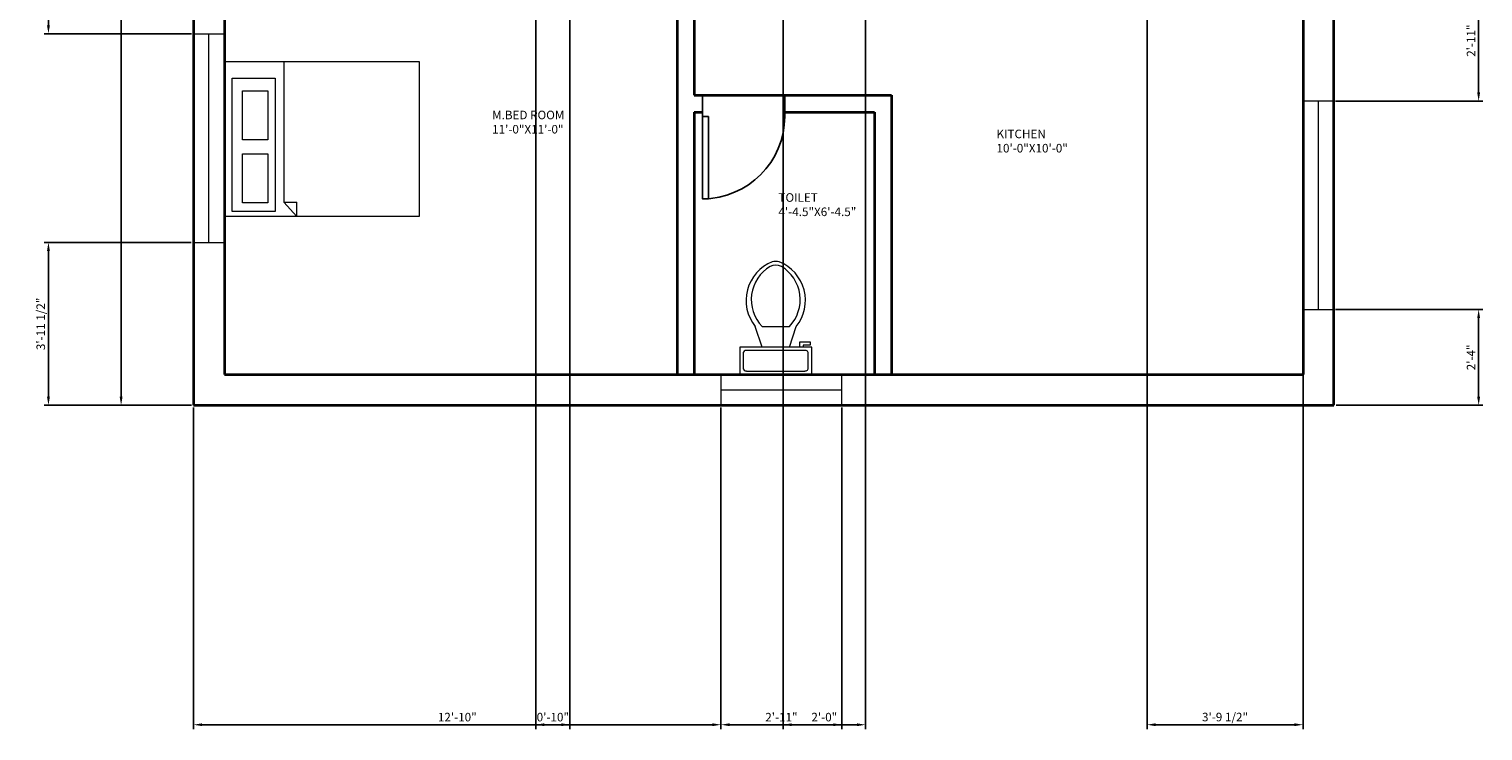
# Model space of a CAD drawing. Units: inches. Extents: x 4673 to 5097, y 7020 to 7947.
# Tile 1 of 3: x 4673 to 5097, y 7020 to 7225. Entities that reach past the tile are written whole.
import ezdxf

# ---------------------------------------------------------------- set-up
doc = ezdxf.new("R2010")
doc.units = ezdxf.units.IN
for name, color, linetype, lineweight in [('A-ANNO-DIMS', 244, 'Continuous', 18), ('A-AREA-IDEN', 7, 'Continuous', 18), ('A-DOOR', 4, 'Continuous', 25), ('A-FLOR-FIXT', 8, 'Continuous', 18), ('A-FURN', 152, 'Continuous', 18), ('A-GLAZ', 152, 'Continuous', 18), ('A-WALL', 7, 'Continuous', 35)]:
    doc.layers.add(name, color=color, linetype=linetype, lineweight=lineweight)
doc.styles.get("Standard").update_dxf_attribs({"font": 'arial.ttf'})
doc.dimstyles.new('ISO-25', dxfattribs={"dimtxt": 2.5, "dimasz": 2.5, "dimexe": 1.25, "dimexo": 0.625, "dimtad": 1, "dimlunit": 3, "dimtxsty": 'Standard', "dimcen": 2.5, "dimadec": 0, "dimazin": 0, "dimtfac": 1, "dimtmove": 0, "dimatfit": 3, "dimfxl": 1, "dimarcsym": 0})

# ---------------------------------------------------------------- blocks, each defined once
blk = doc.blocks.new('*U6')
for p, q in [((-24, 0), (-24, -6)), ((0, 0), (0, -6))]:
    blk.add_line(p, q)
blk.add_lwpolyline([(0, 0), (0, 24), (-1.75, 24), (-1.75, 0)], close=True)
blk.add_arc((0, 0), 24, 90, 180)
blk = doc.blocks.new('*U8')
for p, q in [((9.5, -6), (9.5, -2)), ((-8, -8.5), (-8, -8)), ((-7, -8), (-7, -9.5)), ((-4, -8), (-6, -14)), ((4, -8), (6, -14)), ((-10, -8.5), (-8, -8.5)), ((-10, -9.5), (-10, -8.5)), ((-7, -9.5), (-10, -9.5)), ((4, -14), (-4, -14))]:
    blk.add_line(p, q)
blk.add_lwpolyline([(10.5, -8), (10.5, 0), (-10.5, 0), (-10.5, -8)], close=True)
for points in [[(-9.5, -2), (-9.5, -6)], [(8.5, -1), (-8.5, -1)], [(-8.5, -7), (8.5, -7)]]:
    blk.add_lwpolyline(points)
for centre, radius, start, end in [((-8.62, -1.88), 0.884, 81.8699, 188.1301), ((8.62, -1.88), 0.884, 351.8699, 98.1301), ((-8.62, -6.12), 0.884, 171.8699, 278.1301), ((8.62, -6.12), 0.884, 261.8699, 8.1301), ((3.52, -21.58), 12.17, 141.4691, 247.9714), ((4.2, -21.82), 11.33, 136.3677, 238.9468), ((-3.52, -21.58), 12.17, 292.0284, 38.5307), ((-4.2, -21.82), 11.33, 301.053, 43.6321), ((0, -27.88), 4, 245.7318, 294.2682), ((0, -29), 4, 254.8605, 285.1395)]:
    blk.add_arc(centre, radius, start, end)
blk = doc.blocks.new('*D10')
at = {"layer": 'A-ANNO-DIMS', "color": 0, "lineweight": -2, "transparency": 16777216}
for p, q in [((4720.26, 7847.86), (4698.51, 7847.86)), ((4699.76, 7845.36), (4699.76, 7117.36)), ((4720.26, 7114.86), (4698.51, 7114.86))]:
    blk.add_line(p, q, dxfattribs=at)
at = {"layer": 'A-ANNO-DIMS', "color": 0, "transparency": 16777216}
for points in [[(4699.34, 7845.36), (4700.18, 7845.36), (4699.76, 7847.86)], [(4699.34, 7117.36), (4700.18, 7117.36), (4699.76, 7114.86)]]:
    blk.add_solid(points, dxfattribs=at)
at = {"layer": 'Defpoints', "color": 0, "transparency": 16777216}
for p in [(4720.89, 7847.86), (4699.76, 7114.86), (4720.89, 7114.86)]:
    blk.add_point(p, dxfattribs=at)
at = {"layer": 'A-ANNO-DIMS', "color": 0, "transparency": 16777216, "insert": (4697.86, 7481.36), "char_height": 2.5, "attachment_point": 5, "rotation": 90}
blk.add_mtext('61\'-1"', dxfattribs=at)
blk = doc.blocks.new('BED-DOUBLE')
for p, q in [((17.35, 45.28), (17.35, 4.23)), ((17.35, 4.23), (21.14, 0)), ((17.35, 4.23), (21.14, 4.23)), ((21.14, 0), (21.14, 4.23))]:
    blk.add_line(p, q)
for points in [[(0, 0), (0, 45.28), (56.77, 45.28), (56.77, 0)], [(2.29, 1.5), (2.29, 40.39), (14.79, 40.39), (14.79, 1.5)], [(5.28, 22.37), (5.28, 36.69), (12.64, 36.69), (12.64, 22.37)], [(5.28, 4.03), (5.28, 18.35), (12.64, 18.35), (12.64, 4.03)]]:
    blk.add_lwpolyline(points, close=True)
blk = doc.blocks.new('WIN-61IN')
for p, q in [((9, 60.82), (0, 60.82)), ((0.12, 60.89), (0.12, 0.07)), ((9, 60.82), (4.5, 60.82)), ((4.5, 60.82), (4.5, 0)), ((9.12, 0), (9.12, 60.82)), ((0, 0), (9, 0))]:
    blk.add_line(p, q)
blk = doc.blocks.new('*D23')
at = {"layer": 'A-ANNO-DIMS', "color": 0, "lineweight": -2, "transparency": 16777216}
for p, q in [((4998.89, 7243.24), (4998.89, 7020.41)), ((5044.39, 7243.24), (5044.39, 7020.41)), ((5001.39, 7021.66), (5041.89, 7021.66))]:
    blk.add_line(p, q, dxfattribs=at)
at = {"layer": 'A-ANNO-DIMS', "color": 0, "transparency": 16777216}
for points in [[(5001.39, 7022.08), (5001.39, 7021.25), (4998.89, 7021.66)], [(5041.89, 7022.08), (5041.89, 7021.25), (5044.39, 7021.66)]]:
    blk.add_solid(points, dxfattribs=at)
at = {"layer": 'Defpoints', "color": 0, "transparency": 16777216}
for p in [(4998.89, 7243.86), (5044.39, 7243.86), (5044.39, 7021.66)]:
    blk.add_point(p, dxfattribs=at)
at = {"layer": 'A-ANNO-DIMS', "color": 0, "transparency": 16777216, "insert": (5021.64, 7023.58), "char_height": 2.5, "attachment_point": 5}
blk.add_mtext('3\'-9 1/2"', dxfattribs=at)
blk = doc.blocks.new('*D29')
at = {"layer": 'A-ANNO-DIMS', "color": 0, "lineweight": -2, "transparency": 16777216}
for p, q in [((4874.67, 7114.24), (4874.67, 7020.41)), ((4909.91, 7114.24), (4909.91, 7020.41)), ((4877.17, 7021.66), (4907.41, 7021.66))]:
    blk.add_line(p, q, dxfattribs=at)
at = {"layer": 'A-ANNO-DIMS', "color": 0, "transparency": 16777216}
for points in [[(4877.17, 7022.08), (4877.17, 7021.25), (4874.67, 7021.66)], [(4907.41, 7022.08), (4907.41, 7021.25), (4909.91, 7021.66)]]:
    blk.add_solid(points, dxfattribs=at)
at = {"layer": 'Defpoints', "color": 0, "transparency": 16777216}
for p in [(4874.67, 7114.86), (4909.91, 7114.86), (4909.91, 7021.66)]:
    blk.add_point(p, dxfattribs=at)
at = {"layer": 'A-ANNO-DIMS', "color": 0, "transparency": 16777216, "insert": (4892.29, 7023.54), "char_height": 2.5, "attachment_point": 5}
blk.add_mtext('2\'-11"', dxfattribs=at)
blk = doc.blocks.new('*D30')
at = {"layer": 'A-ANNO-DIMS', "color": 0, "lineweight": -2, "transparency": 16777216}
for p, q in [((4720.89, 7114.24), (4720.89, 7020.41)), ((4874.67, 7114.24), (4874.67, 7020.41)), ((4723.39, 7021.66), (4872.17, 7021.66))]:
    blk.add_line(p, q, dxfattribs=at)
at = {"layer": 'A-ANNO-DIMS', "color": 0, "transparency": 16777216}
for points in [[(4723.39, 7022.08), (4723.39, 7021.25), (4720.89, 7021.66)], [(4872.17, 7022.08), (4872.17, 7021.25), (4874.67, 7021.66)]]:
    blk.add_solid(points, dxfattribs=at)
at = {"layer": 'Defpoints', "color": 0, "transparency": 16777216}
for p in [(4720.89, 7114.86), (4874.67, 7114.86), (4874.67, 7021.66)]:
    blk.add_point(p, dxfattribs=at)
at = {"layer": 'A-ANNO-DIMS', "color": 0, "transparency": 16777216, "insert": (4797.78, 7023.56), "char_height": 2.5, "attachment_point": 5}
blk.add_mtext('12\'-10"', dxfattribs=at)
blk = doc.blocks.new('*D33')
at = {"layer": 'A-ANNO-DIMS', "color": 0, "lineweight": -2, "transparency": 16777216}
for p, q in [((4820.64, 7490.24), (4820.64, 7020.41)), ((4830.64, 7490.24), (4830.64, 7020.41)), ((4823.14, 7021.66), (4828.14, 7021.66))]:
    blk.add_line(p, q, dxfattribs=at)
at = {"layer": 'A-ANNO-DIMS', "color": 0, "transparency": 16777216}
for points in [[(4823.14, 7022.08), (4823.14, 7021.25), (4820.64, 7021.66)], [(4828.14, 7022.08), (4828.14, 7021.25), (4830.64, 7021.66)]]:
    blk.add_solid(points, dxfattribs=at)
at = {"layer": 'Defpoints', "color": 0, "transparency": 16777216}
for p in [(4820.64, 7490.86), (4830.64, 7490.86), (4830.64, 7021.66)]:
    blk.add_point(p, dxfattribs=at)
at = {"layer": 'A-ANNO-DIMS', "color": 0, "transparency": 16777216, "insert": (4825.64, 7023.56), "char_height": 2.5, "attachment_point": 5}
blk.add_mtext('0\'-10"', dxfattribs=at)
blk = doc.blocks.new('*D35')
at = {"layer": 'A-ANNO-DIMS', "color": 0, "lineweight": -2, "transparency": 16777216}
for p, q in [((4892.8, 7756.68), (4892.8, 7020.41)), ((4916.8, 7756.68), (4916.8, 7020.41)), ((4895.3, 7021.66), (4914.3, 7021.66))]:
    blk.add_line(p, q, dxfattribs=at)
at = {"layer": 'A-ANNO-DIMS', "color": 0, "transparency": 16777216}
for points in [[(4895.3, 7022.08), (4895.3, 7021.25), (4892.8, 7021.66)], [(4914.3, 7022.08), (4914.3, 7021.25), (4916.8, 7021.66)]]:
    blk.add_solid(points, dxfattribs=at)
at = {"layer": 'Defpoints', "color": 0, "transparency": 16777216}
for p in [(4892.8, 7757.31), (4916.8, 7757.31), (4916.8, 7021.66)]:
    blk.add_point(p, dxfattribs=at)
at = {"layer": 'A-ANNO-DIMS', "color": 0, "transparency": 16777216, "insert": (4904.8, 7023.56), "char_height": 2.5, "attachment_point": 5}
blk.add_mtext('2\'-0"', dxfattribs=at)
blk = doc.blocks.new('*D36')
at = {"layer": 'A-ANNO-DIMS', "color": 0, "lineweight": -2, "transparency": 16777216}
for p, q in [((4720.14, 7162.36), (4677.32, 7162.36)), ((4678.57, 7117.36), (4678.57, 7159.86)), ((4720.26, 7114.86), (4677.32, 7114.86))]:
    blk.add_line(p, q, dxfattribs=at)
at = {"layer": 'A-ANNO-DIMS', "color": 0, "transparency": 16777216}
for points in [[(4678.15, 7159.86), (4678.99, 7159.86), (4678.57, 7162.36)], [(4678.15, 7117.36), (4678.99, 7117.36), (4678.57, 7114.86)]]:
    blk.add_solid(points, dxfattribs=at)
at = {"layer": 'Defpoints', "color": 0, "transparency": 16777216}
for p in [(4678.57, 7162.36), (4720.77, 7162.36), (4720.89, 7114.86)]:
    blk.add_point(p, dxfattribs=at)
at = {"layer": 'A-ANNO-DIMS', "color": 0, "transparency": 16777216, "insert": (4676.65, 7138.61), "char_height": 2.5, "attachment_point": 5, "rotation": 90}
blk.add_mtext('3\'-11 1/2"', dxfattribs=at)
blk = doc.blocks.new('*D37')
at = {"layer": 'A-ANNO-DIMS', "color": 0, "lineweight": -2, "transparency": 16777216}
for p, q in [((4729.26, 7250.86), (4677.32, 7250.86)), ((4678.57, 7225.75), (4678.57, 7248.36)), ((4720.26, 7223.25), (4677.32, 7223.25))]:
    blk.add_line(p, q, dxfattribs=at)
at = {"layer": 'A-ANNO-DIMS', "color": 0, "transparency": 16777216}
for points in [[(4678.15, 7248.36), (4678.99, 7248.36), (4678.57, 7250.86)], [(4678.15, 7225.75), (4678.99, 7225.75), (4678.57, 7223.25)]]:
    blk.add_solid(points, dxfattribs=at)
at = {"layer": 'Defpoints', "color": 0, "transparency": 16777216}
for p in [(4678.57, 7250.86), (4729.89, 7250.86), (4720.89, 7223.25)]:
    blk.add_point(p, dxfattribs=at)
at = {"layer": 'A-ANNO-DIMS', "color": 0, "transparency": 16777216, "insert": (4676.65, 7237.05), "char_height": 2.5, "attachment_point": 5, "rotation": 90}
blk.add_mtext('2\'-3 1/2"', dxfattribs=at)
blk = doc.blocks.new('*D43')
at = {"layer": 'A-ANNO-DIMS', "color": 0, "lineweight": -2, "transparency": 16777216}
for p, q in [((5053.89, 7142.81), (5096.84, 7142.81)), ((5095.59, 7117.36), (5095.59, 7140.31)), ((5054.01, 7114.86), (5096.84, 7114.86))]:
    blk.add_line(p, q, dxfattribs=at)
at = {"layer": 'A-ANNO-DIMS', "color": 0, "transparency": 16777216}
for points in [[(5095.17, 7140.31), (5096.01, 7140.31), (5095.59, 7142.81)], [(5095.17, 7117.36), (5096.01, 7117.36), (5095.59, 7114.86)]]:
    blk.add_solid(points, dxfattribs=at)
at = {"layer": 'Defpoints', "color": 0, "transparency": 16777216}
for p in [(5053.27, 7142.81), (5095.59, 7142.81), (5053.39, 7114.86)]:
    blk.add_point(p, dxfattribs=at)
at = {"layer": 'A-ANNO-DIMS', "color": 0, "transparency": 16777216, "insert": (5093.71, 7128.84), "char_height": 2.5, "attachment_point": 5, "rotation": 90}
blk.add_mtext('2\'-4"', dxfattribs=at)
blk = doc.blocks.new('*D44')
at = {"layer": 'A-ANNO-DIMS', "color": 0, "lineweight": -2, "transparency": 16777216}
for p, q in [((5045.01, 7238.86), (5096.84, 7238.86)), ((5095.59, 7206.13), (5095.59, 7236.36)), ((5053.89, 7203.63), (5096.84, 7203.63))]:
    blk.add_line(p, q, dxfattribs=at)
at = {"layer": 'A-ANNO-DIMS', "color": 0, "transparency": 16777216}
for points in [[(5095.17, 7236.36), (5096.01, 7236.36), (5095.59, 7238.86)], [(5095.17, 7206.13), (5096.01, 7206.13), (5095.59, 7203.63)]]:
    blk.add_solid(points, dxfattribs=at)
at = {"layer": 'Defpoints', "color": 0, "transparency": 16777216}
for p in [(5044.39, 7238.86), (5095.59, 7238.86), (5053.27, 7203.63)]:
    blk.add_point(p, dxfattribs=at)
at = {"layer": 'A-ANNO-DIMS', "color": 0, "transparency": 16777216, "insert": (5093.71, 7221.25), "char_height": 2.5, "attachment_point": 5, "rotation": 90}
blk.add_mtext('2\'-11"', dxfattribs=at)

msp = doc.modelspace()

# ---------------------------------------------------------------- linework, layer by layer
at = {"layer": 'A-GLAZ'}
for p, q in [((5053.269, 7203.63), (5044.269, 7203.63)), ((5044.269, 7203.63), (5044.269, 7142.812)), ((5053.269, 7203.63), (5048.769, 7203.63)), ((5048.769, 7203.63), (5048.769, 7142.812)), ((5053.269, 7142.812), (5053.269, 7203.63)), ((5044.269, 7142.812), (5053.269, 7142.812)), ((4874.666, 7123.863), (4874.666, 7114.863)), ((4909.91, 7123.863), (4874.666, 7123.863)), ((4874.666, 7123.863), (4874.666, 7119.363)), ((4909.91, 7114.863), (4909.91, 7123.863)), ((4874.666, 7119.363), (4909.91, 7119.363)), ((4874.666, 7114.863), (4909.91, 7114.863))]:
    msp.add_line(p, q, dxfattribs=at)
at = {"layer": 'A-WALL'}
for p, q in [((4720.889, 7847.863), (4720.889, 7114.863)), ((5053.389, 7114.863), (5053.389, 7293.326)), ((4866.889, 7255.863), (4866.889, 7205.363)), ((4729.889, 7250.863), (4729.889, 7123.863)), ((4861.889, 7250.863), (4861.889, 7123.863)), ((5044.389, 7238.863), (5044.389, 7123.863)), ((4866.889, 7205.363), (4924.389, 7205.363)), ((4924.389, 7205.363), (4924.389, 7123.863)), ((4866.889, 7200.363), (4869.264, 7200.363)), ((4866.889, 7200.363), (4866.889, 7123.863)), ((4893.264, 7200.363), (4919.389, 7200.363)), ((4919.389, 7200.363), (4919.389, 7123.863)), ((4729.889, 7123.863), (4861.889, 7123.863)), ((4861.889, 7123.863), (4919.389, 7123.863)), ((4919.389, 7123.863), (5044.389, 7123.863)), ((4720.889, 7114.863), (4866.889, 7114.863)), ((4866.889, 7114.863), (5053.389, 7114.863))]:
    msp.add_line(p, q, dxfattribs=at)

# ---------------------------------------------------------------- block references
at = {"layer": 'A-DOOR', "rotation": 180}
msp.add_blockref('*U6', (4869.264, 7199.116), dxfattribs=at)
at = {"layer": 'A-FLOR-FIXT', "rotation": 180}
msp.add_blockref('*U8', (4890.639, 7123.863), dxfattribs=at)
at = {"layer": 'A-FURN'}
msp.add_blockref('BED-DOUBLE', (4729.889, 7169.899), dxfattribs=at)
at = {"layer": 'A-GLAZ'}
msp.add_blockref('WIN-61IN', (4720.769, 7162.36), dxfattribs=at)

# ---------------------------------------------------------------- texts
at = {"layer": 'A-AREA-IDEN', "char_height": 2.5, "attachment_point": 1}
for s, width, insert in [('M.BED ROOM\\P11\'-0"X11\'-0"', 39.07245, (4807.934, 7200.812)), ('KITCHEN\\P10\'-0"X10\'-0"', 42.37167, (4955.002, 7195.289)), ('TOILET\\P4\'-4.5"X6\'-4.5"', 15.51522, (4891.426, 7176.734))]:
    msp.add_mtext_dynamic_manual_height_columns(s, width=width, gutter_width=12.5, heights=[0], dxfattribs=dict(at, insert=insert))

# ---------------------------------------------------------------- dimensions: what is measured, and where the dimension line sits
at = {"layer": 'A-ANNO-DIMS'}
for base, p1, p2, override, picture, middle in [((4699.76, 7114.863), (4720.889, 7847.863), (4720.889, 7114.863), {"dimclrd": 0, "dimclre": 0, "dimclrt": 0}, '*D10', (4697.858, 7481.363)), ((4678.569, 7250.863), (4720.889, 7223.246), (4729.889, 7250.863), {"dimdec": 1, "dimlfac": 1, "dimrnd": 0, "dimzin": 1, "dimdsep": 46, "dimlunit": 4, "dimfrac": 2}, '*D37', (4676.651, 7237.054)), ((5095.589, 7238.863), (5053.269, 7203.63), (5044.389, 7238.863), {"dimdec": 1, "dimlfac": 1, "dimrnd": 0, "dimzin": 1, "dimdsep": 46, "dimlunit": 4, "dimfrac": 2}, '*D44', (5093.708, 7221.246)), ((4678.569, 7162.36), (4720.889, 7114.863), (4720.769, 7162.36), {"dimdec": 1, "dimlfac": 1, "dimrnd": 0, "dimzin": 1, "dimdsep": 46, "dimlunit": 4, "dimfrac": 2}, '*D36', (4676.651, 7138.611)), ((5095.5886, 7142.8125), (5053.3886, 7114.8629), (5053.2694, 7142.8125), {"dimdec": 1, "dimlfac": 1, "dimrnd": 0, "dimzin": 1, "dimdsep": 46, "dimlunit": 4, "dimfrac": 2}, '*D43', (5093.7085, 7128.8377))]:
    dim = msp.add_linear_dim(base=base, p1=p1, p2=p2, angle=90, dimstyle='ISO-25', override=override, dxfattribs=at)
    dim.commit()
    dim.dimension.update_dxf_attribs({"geometry": picture, "text_midpoint": middle})
for base, p1, p2, picture, middle in [((4916.804, 7021.663), (4892.804, 7757.308), (4916.804, 7757.308), '*D35', (4904.804, 7023.564)), ((4830.639, 7021.663), (4820.639, 7490.863), (4830.639, 7490.863), '*D33', (4825.639, 7023.564)), ((5044.389, 7021.663), (4998.889, 7243.863), (5044.389, 7243.863), '*D23', (5021.639, 7023.581)), ((4874.666, 7021.663), (4720.889, 7114.863), (4874.666, 7114.863), '*D30', (4797.777, 7023.564)), ((4909.91, 7021.663), (4874.666, 7114.863), (4909.91, 7114.863), '*D29', (4892.288, 7023.543))]:
    dim = msp.add_linear_dim(base=base, p1=p1, p2=p2, dimstyle='ISO-25', override={"dimdec": 1, "dimlfac": 1, "dimrnd": 0, "dimzin": 1, "dimdsep": 46, "dimlunit": 4, "dimfrac": 2}, dxfattribs=at)
    dim.commit()
    dim.dimension.update_dxf_attribs({"geometry": picture, "text_midpoint": middle})

doc.saveas('drawing.dxf')
